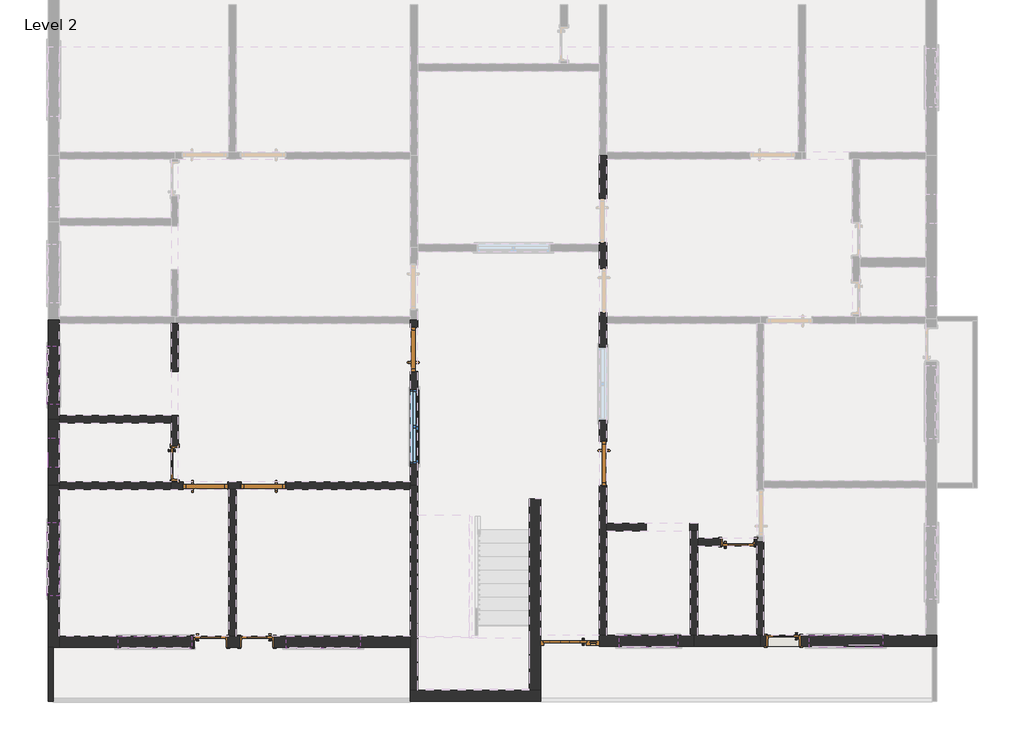
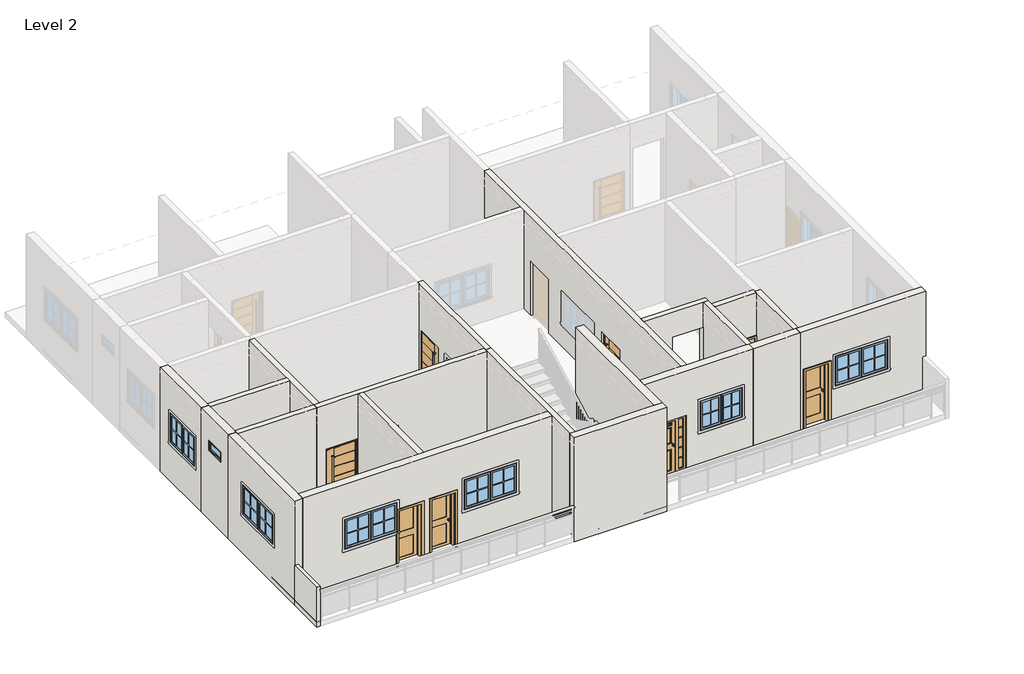
# One storey, part 1 of 5: 22 walls, 10 doors, 8 windows.
"""IFC4 building model written with IfcOpenShell, lengths in millimetres."""

from ifc_helpers import new_model, si_unit, frame, origin, place, context, project, spatial, polyline, outline, extrude, faceted_brep, transform, mapped, element, save
from components import door_3_ad1505b7, door_3_44036f4b, extsgl_w_side_panel_4_38b62cc9, door_c5a180fb, door_5f4ff63b, door_e2914254, fixed_2_d9cafb20, m_window_awning_double_horizontal_4_0c6a2509, m_window_awning_double_horizontal_5_7c720334, m_window_awning_double_horizontal_5_337400f2

model = new_model("IFC4")

# Units and contexts
model_context = context("Model", 3, world=origin())
ifc_project = project(units=[si_unit("LENGTHUNIT", "METRE", prefix="MILLI")], contexts=[model_context])

# Site, building, storey
site = spatial("IfcSite", under=ifc_project)
building = spatial("IfcBuilding", under=site)
storey = spatial("IfcBuildingStorey", under=building, Name="Level 2", Elevation=3200.4)

# Doors
placement = place(None, origin())
door_3_shape = door_3_ad1505b7(model_context)
element("IfcDoor", 1, ObjectType="3'", at=placement, inside=storey, context=model_context, shape_type="MappedRepresentation", body=[
    mapped(door_3_shape, transform((-17435.4847893, 15964.9922903, 3200.4), x_axis=(0.0, 1.0, 0.0), y_axis=(-1.0, 0.0, 0.0), z_axis=(0.0, 0.0, 1.0))),
])
element("IfcDoor", 2, ObjectType="3'", at=placement, inside=storey, context=model_context, shape_type="MappedRepresentation", body=[
    mapped(door_3_shape, transform((-20559.6847893, 13145.5922903, 3200.4), x_axis=(-1.0, 0.0, 0.0), y_axis=(0.0, -1.0, 0.0), z_axis=(0.0, 0.0, 1.0))),
])
element("IfcDoor", 3, ObjectType="3'", at=placement, inside=storey, context=model_context, shape_type="MappedRepresentation", body=[
    mapped(door_3_shape, transform((-13523.8847893, 13602.7922903, 3200.4), x_axis=(0.0, -1.0, 0.0), y_axis=(1.0, 0.0, 0.0), z_axis=(0.0, 0.0, 1.0))),
])
door_3_2_shape = door_3_44036f4b(model_context)
element("IfcDoor", 4, ObjectType="3'", at=placement, inside=storey, context=model_context, shape_type="MappedRepresentation", body=[
    mapped(door_3_2_shape, transform((-21753.4847893, 13145.5922903, 3200.4), x_axis=(1.0, 0.0, 0.0), y_axis=(0.0, 1.0, 0.0), z_axis=(0.0, 0.0, 1.0))),
])
extsgl_w_side_panel_4_shape = extsgl_w_side_panel_4_38b62cc9(model_context)
element("IfcDoor", 5, ObjectType="ExtSgl w Side Panel : 4'", at=placement, inside=storey, context=model_context, shape_type="MappedRepresentation", body=[
    mapped(extsgl_w_side_panel_4_shape, transform((-14429.0847893, 9932.4922903, 3200.4), x_axis=(-1.0, 0.0, 0.0), y_axis=(0.0, -1.0, 0.0), z_axis=(0.0, 0.0, 1.0))),
])
door_shape = door_c5a180fb(model_context)
element("IfcDoor", 6, ObjectType="M_Door-Interior-Single-2_Panel-Wood : 2'2\"", at=placement, inside=storey, context=model_context, shape_type="MappedRepresentation", body=[
    mapped(door_shape, transform((-22391.6597893, 13602.7922903, 3200.4), x_axis=(0.0, -1.0, 0.0), y_axis=(1.0, 0.0, 0.0), z_axis=(0.0, 0.0, 1.0))),
])
element("IfcDoor", 7, ObjectType="M_Door-Interior-Single-2_Panel-Wood : 2'2\"", at=placement, inside=storey, context=model_context, shape_type="MappedRepresentation", body=[
    mapped(door_shape, transform((-10729.8847893, 11974.0172903, 3200.4), x_axis=(1.0, 0.0, 0.0), y_axis=(0.0, 1.0, 0.0), z_axis=(0.0, 0.0, 1.0))),
])
door_2_shape = door_5f4ff63b(model_context)
element("IfcDoor", 8, ObjectType="M_Door-Interior-Single-2_Panel-Wood : 2'2\"", at=placement, inside=storey, context=model_context, shape_type="MappedRepresentation", body=[
    mapped(door_2_shape, transform((-21651.8847893, 9910.2672903, 3200.4), x_axis=(1.0, 0.0, 0.0), y_axis=(0.0, 1.0, 0.0), z_axis=(0.0, 0.0, 1.0))),
])
door_4_shape = door_e2914254(model_context)
element("IfcDoor", 9, ObjectType="M_Door-Interior-Single-2_Panel-Wood : 2'2\"", at=placement, inside=storey, context=model_context, shape_type="MappedRepresentation", body=[
    mapped(door_4_shape, transform((-20686.6847893, 9910.2672903, 3200.4), x_axis=(-1.0, 0.0, 0.0), y_axis=(0.0, -1.0, 0.0), z_axis=(0.0, 0.0, 1.0))),
])
element("IfcDoor", 10, ObjectType="M_Door-Interior-Single-2_Panel-Wood : 2'2\"", at=placement, inside=storey, context=model_context, shape_type="MappedRepresentation", body=[
    mapped(door_4_shape, transform((-9790.0847893, 9935.6672903, 3352.8), x_axis=(-1.0, 0.0, 0.0), y_axis=(0.0, -1.0, 0.0), z_axis=(0.0, 0.0, 1.0))),
])

# Walls
element("IfcWall", 11, ObjectType="Generic - 4\"", at=placement, inside=storey, context=model_context, shape_type="SweptSolid", body=[
    extrude(outline(polyline([(-25004.6847893, 8675.1922903), (-25004.6847893, 9792.7922903), (-24903.0847893, 9792.7922903), (-24903.0847893, 8675.1922903), (-25004.6847893, 8675.1922903)])), frame((0.0, 0.0, 3200.4), z_axis=(0.0, 0.0, 1.0), x_axis=(1.0, 0.0, 0.0)), (0.0, 0.0, 1.0), 1219.2),
])
element("IfcWall", 12, ObjectType="Generic - 6\"", at=placement, inside=storey, context=model_context, shape_type="Brep", body=[
    faceted_brep([(-24776.0847893, 13069.3922903, 3200.4), (-22477.3847893, 13069.3922903, 3200.4), (-22477.3847893, 13069.3922903, 6400.8), (-24776.0847893, 13069.3922903, 6400.8), (-24776.0847893, 13221.7922903, 3200.4), (-24776.0847893, 13221.7922903, 6400.8), (-22477.3847893, 13221.7922903, 6400.8), (-22477.3847893, 13221.7922903, 3200.4), (-24776.0847893, 13145.5922903, 3200.4), (-24776.0847893, 13145.5922903, 6400.8)], [[[0, 1, 2, 3]], [[4, 5, 6, 7]], [[1, 0, 8, 4, 7]], [[2, 1, 7, 6]], [[3, 2, 6, 5, 9]], [[0, 3, 9, 5, 4, 8]]]),
])
element("IfcWall", 13, ObjectType="Generic - 6\"", at=placement, inside=storey, context=model_context, shape_type="Brep", body=[
    faceted_brep([(-22464.6847893, 13221.7922903, 6400.8), (-22464.6847893, 14440.9922903, 6400.8), (-22464.6847893, 14593.3922903, 6400.8), (-22464.6847893, 16498.3922903, 6400.8), (-22464.6847893, 16498.3922903, 3200.4), (-22464.6847893, 15507.100075, 3200.4), (-22464.6847893, 15507.100075, 5638.8), (-22464.6847893, 14599.1617976, 5638.8), (-22464.6847893, 14599.1617976, 3200.4), (-22464.6847893, 14593.3922903, 3200.4), (-22464.6847893, 14440.9922903, 3200.4), (-22464.6847893, 13957.9922903, 3200.4), (-22464.6847893, 13957.9922903, 5054.2), (-22464.6847893, 13247.5922903, 5054.2), (-22464.6847893, 13247.5922903, 3200.4), (-22464.6847893, 13221.7922903, 3200.4), (-22312.2847893, 16498.3922903, 6400.8), (-22312.2847893, 13221.7922903, 6400.8), (-22312.2847893, 13221.7922903, 3200.4), (-22312.2847893, 13247.5922903, 3200.4), (-22312.2847893, 13247.5922903, 5054.2), (-22312.2847893, 13957.9922903, 5054.2), (-22312.2847893, 13957.9922903, 3200.4), (-22312.2847893, 14599.1617976, 3200.4), (-22312.2847893, 14599.1617976, 5638.8), (-22312.2847893, 15507.100075, 5638.8), (-22312.2847893, 15507.100075, 3200.4), (-22312.2847893, 16498.3922903, 3200.4), (-22388.4847893, 16498.3922903, 3200.4), (-22388.4847893, 16498.3922903, 6400.8)], [[[0, 1, 2, 3, 4, 5, 6, 7, 8, 9, 10, 11, 12, 13, 14, 15]], [[16, 17, 18, 19, 20, 21, 22, 23, 24, 25, 26, 27]], [[18, 15, 14, 19]], [[8, 23, 22, 11, 10, 9]], [[4, 28, 27, 26, 5]], [[3, 2, 1, 0, 17, 16, 29]], [[4, 3, 29, 16, 27, 28]], [[0, 15, 18, 17]], [[13, 20, 19, 14]], [[20, 13, 12, 21]], [[21, 12, 11, 22]], [[6, 25, 24, 7]], [[25, 6, 5, 26]], [[7, 24, 23, 8]]]),
])
element("IfcWall", 14, ObjectType="Generic - 6\"", at=placement, inside=storey, context=model_context, shape_type="Brep", body=[
    faceted_brep([(-24776.0847893, 14440.9922903, 3200.4), (-22464.6847893, 14440.9922903, 3200.4), (-22464.6847893, 14440.9922903, 6400.8), (-24776.0847893, 14440.9922903, 6400.8), (-24776.0847893, 14593.3922903, 3200.4), (-24776.0847893, 14593.3922903, 6400.8), (-22464.6847893, 14593.3922903, 6400.8), (-22464.6847893, 14593.3922903, 3200.4), (-24776.0847893, 14517.1922903, 3200.4), (-24776.0847893, 14517.1922903, 6400.8)], [[[0, 1, 2, 3]], [[4, 5, 6, 7]], [[1, 0, 8, 4, 7]], [[3, 2, 6, 5, 9]], [[0, 3, 9, 5, 4, 8]], [[2, 1, 7, 6]]]),
])
element("IfcWall", 15, ObjectType="Generic - 6\"", at=placement, inside=storey, context=model_context, shape_type="SweptSolid", body=[
    extrude(outline(polyline([(-21118.4847893, 13069.3922903), (-21118.4847893, 10021.3922903), (-21270.8847893, 10021.3922903), (-21270.8847893, 13069.3922903), (-21118.4847893, 13069.3922903)])), frame((0.0, 0.0, 3200.4), z_axis=(0.0, 0.0, 1.0), x_axis=(1.0, 0.0, 0.0)), (0.0, 0.0, 1.0), 3200.4),
])
element("IfcWall", 16, ObjectType="Generic - 6\"", at=placement, inside=storey, context=model_context, shape_type="Brep", body=[
    faceted_brep([(-11568.0847893, 12205.7922903, 3200.4), (-11568.0847893, 12205.7922903, 6400.8), (-11720.4847893, 12205.7922903, 6400.8), (-13447.6847893, 12205.7922903, 6400.8), (-13447.6847893, 12205.7922903, 3200.4), (-12628.6631671, 12205.7922903, 3200.4), (-12628.6631671, 12205.7922903, 5638.8), (-11726.8987952, 12205.7922903, 5638.8), (-11726.8987952, 12205.7922903, 3200.4), (-11720.4847893, 12205.7922903, 3200.4), (-11568.0847893, 12358.1922903, 6400.8), (-11568.0847893, 12358.1922903, 3200.4), (-11726.8987952, 12358.1922903, 3200.4), (-11726.8987952, 12358.1922903, 5638.8), (-12628.6631671, 12358.1922903, 5638.8), (-12628.6631671, 12358.1922903, 3200.4), (-13447.6847893, 12358.1922903, 3200.4), (-13447.6847893, 12358.1922903, 6400.8)], [[[0, 1, 2, 3, 4, 5, 6, 7, 8, 9]], [[10, 11, 12, 13, 14, 15, 16, 17]], [[4, 16, 15, 5]], [[11, 0, 9, 8, 12]], [[3, 2, 1, 10, 17]], [[4, 3, 17, 16]], [[1, 0, 11, 10]], [[6, 14, 13, 7]], [[14, 6, 5, 15]], [[7, 13, 12, 8]]]),
])
element("IfcWall", 17, ObjectType="Generic - 6\"", at=placement, inside=storey, context=model_context, shape_type="Brep", body=[
    faceted_brep([(-11720.4847893, 12205.7922903, 3200.4), (-11720.4847893, 10046.7922903, 3200.4), (-11720.4847893, 10046.7922903, 6400.8), (-11720.4847893, 12205.7922903, 6400.8), (-11568.0847893, 12205.7922903, 3200.4), (-11568.0847893, 12205.7922903, 6400.8), (-11568.0847893, 12053.3922903, 6400.8), (-11568.0847893, 11900.9922903, 6400.8), (-11568.0847893, 10046.7922903, 6400.8), (-11568.0847893, 10046.7922903, 3200.4), (-11568.0847893, 11900.9922903, 3200.4), (-11568.0847893, 12053.3922903, 3200.4), (-11644.2847893, 10046.7922903, 3200.4), (-11644.2847893, 10046.7922903, 6400.8)], [[[0, 1, 2, 3]], [[4, 5, 6, 7, 8, 9, 10, 11]], [[1, 0, 4, 11, 10, 9, 12]], [[3, 2, 13, 8, 7, 6, 5]], [[0, 3, 5, 4]], [[2, 1, 12, 9, 8, 13]]]),
])
element("IfcWall", 18, ObjectType="Generic - 6\"", at=placement, inside=storey, context=model_context, shape_type="Brep", body=[
    faceted_brep([(-10348.8847893, 11900.9922903, 6400.8), (-11568.0847893, 11900.9922903, 6400.8), (-11568.0847893, 11900.9922903, 3200.4), (-11085.0847893, 11900.9922903, 3200.4), (-11085.0847893, 11900.9922903, 5054.2), (-10374.6847893, 11900.9922903, 5054.2), (-10374.6847893, 11900.9922903, 3200.4), (-10348.8847893, 11900.9922903, 3200.4), (-11568.0847893, 12053.3922903, 6400.8), (-10348.8847893, 12053.3922903, 6400.8), (-10348.8847893, 12053.3922903, 3200.4), (-10374.6847893, 12053.3922903, 3200.4), (-10374.6847893, 12053.3922903, 5054.2), (-11085.0847893, 12053.3922903, 5054.2), (-11085.0847893, 12053.3922903, 3200.4), (-11568.0847893, 12053.3922903, 3200.4), (-10348.8847893, 11977.1922903, 3200.4), (-10348.8847893, 11977.1922903, 6400.8)], [[[0, 1, 2, 3, 4, 5, 6, 7]], [[8, 9, 10, 11, 12, 13, 14, 15]], [[2, 15, 14, 3]], [[10, 16, 7, 6, 11]], [[1, 0, 17, 9, 8]], [[2, 1, 8, 15]], [[5, 12, 11, 6]], [[12, 5, 4, 13]], [[13, 4, 3, 14]], [[0, 7, 16, 10, 9, 17]]]),
])
element("IfcWall", 19, ObjectType="Generic - 6\"", at=placement, inside=storey, context=model_context, shape_type="Brep", body=[
    faceted_brep([(-13600.0847893, 10046.7922903, 6400.8), (-13600.0847893, 17996.9922903, 6400.8), (-13600.0847893, 18149.3922903, 6400.8), (-13600.0847893, 19978.1922903, 6400.8), (-13600.0847893, 19978.1922903, 3200.4), (-13600.0847893, 19089.1922903, 3200.4), (-13600.0847893, 19089.1922903, 5029.2), (-13600.0847893, 18174.7922903, 5029.2), (-13600.0847893, 18174.7922903, 3200.4), (-13600.0847893, 18149.3922903, 3200.4), (-13600.0847893, 17996.9922903, 3200.4), (-13600.0847893, 17641.3922903, 3200.4), (-13600.0847893, 17641.3922903, 5029.2), (-13600.0847893, 16726.9922903, 5029.2), (-13600.0847893, 16726.9922903, 3200.4), (-13600.0847893, 14059.9922903, 3200.4), (-13600.0847893, 14059.9922903, 5029.2), (-13600.0847893, 13145.5922903, 5029.2), (-13600.0847893, 13145.5922903, 3200.4), (-13600.0847893, 10046.7922903, 3200.4), (-13600.0847893, 10046.7922903, 5029.2), (-13600.0847893, 16015.7922903, 5014.8), (-13600.0847893, 14491.7922903, 5014.8), (-13600.0847893, 14491.7922903, 4100.4), (-13600.0847893, 16015.7922903, 4100.4), (-13447.6847893, 19978.1922903, 6400.8), (-13447.6847893, 19901.9922903, 6400.8), (-13447.6847893, 16650.7922903, 6400.8), (-13447.6847893, 16498.3922903, 6400.8), (-13447.6847893, 12358.1922903, 6400.8), (-13447.6847893, 12205.7922903, 6400.8), (-13447.6847893, 10046.7922903, 6400.8), (-13447.6847893, 10046.7922903, 3200.4), (-13447.6847893, 12205.7922903, 3200.4), (-13447.6847893, 12358.1922903, 3200.4), (-13447.6847893, 13145.5922903, 3200.4), (-13447.6847893, 13145.5922903, 5029.2), (-13447.6847893, 14059.9922903, 5029.2), (-13447.6847893, 14059.9922903, 3200.4), (-13447.6847893, 16498.3922903, 3200.4), (-13447.6847893, 16650.7922903, 3200.4), (-13447.6847893, 16726.9922903, 3200.4), (-13447.6847893, 16726.9922903, 5029.2), (-13447.6847893, 17641.3922903, 5029.2), (-13447.6847893, 17641.3922903, 3200.4), (-13447.6847893, 18174.7922903, 3200.4), (-13447.6847893, 18174.7922903, 5029.2), (-13447.6847893, 19089.1922903, 5029.2), (-13447.6847893, 19089.1922903, 3200.4), (-13447.6847893, 19901.9922903, 3200.4), (-13447.6847893, 19978.1922903, 3200.4), (-13447.6847893, 16015.7922903, 5014.8), (-13447.6847893, 16015.7922903, 4100.4), (-13447.6847893, 14491.7922903, 4100.4), (-13447.6847893, 14491.7922903, 5014.8), (-13544.6847893, 13145.5922903, 3200.4), (-13544.6847893, 13130.5922903, 3200.4), (-13467.6847893, 13130.5922903, 3200.4), (-13467.6847893, 13145.5922903, 3200.4), (-13544.6847893, 14059.9922903, 3200.4), (-13544.6847893, 16726.9922903, 3200.4), (-13544.6847893, 16711.9922903, 3200.4), (-13467.6847893, 16711.9922903, 3200.4), (-13467.6847893, 16726.9922903, 3200.4), (-13467.6847893, 14059.9922903, 3200.4), (-13467.6847893, 14074.9922903, 3200.4), (-13544.6847893, 14074.9922903, 3200.4), (-13544.6847893, 17641.3922903, 3200.4), (-13580.0847893, 18174.7922903, 3200.4), (-13580.0847893, 18159.7922903, 3200.4), (-13503.0847893, 18159.7922903, 3200.4), (-13503.0847893, 18174.7922903, 3200.4), (-13467.6847893, 17641.3922903, 3200.4), (-13467.6847893, 17656.3922903, 3200.4), (-13544.6847893, 17656.3922903, 3200.4), (-13503.0847893, 19089.1922903, 3200.4), (-13503.0847893, 19104.1922903, 3200.4), (-13580.0847893, 19104.1922903, 3200.4), (-13580.0847893, 19089.1922903, 3200.4), (-13544.6847893, 14059.9922903, 5029.2), (-13544.6847893, 13145.5922903, 5029.2), (-13467.6847893, 14059.9922903, 5029.2), (-13467.6847893, 13145.5922903, 5029.2), (-13467.6847893, 14074.9922903, 5044.2), (-13467.6847893, 13130.5922903, 5044.2), (-13544.6847893, 13130.5922903, 5044.2), (-13544.6847893, 14074.9922903, 5044.2), (-13544.6847893, 17641.3922903, 5029.2), (-13544.6847893, 16726.9922903, 5029.2), (-13467.6847893, 17641.3922903, 5029.2), (-13467.6847893, 16726.9922903, 5029.2), (-13467.6847893, 17656.3922903, 5044.2), (-13467.6847893, 16711.9922903, 5044.2), (-13544.6847893, 16711.9922903, 5044.2), (-13544.6847893, 17656.3922903, 5044.2), (-13580.0847893, 19089.1922903, 5029.2), (-13580.0847893, 18174.7922903, 5029.2), (-13503.0847893, 18174.7922903, 5029.2), (-13503.0847893, 19089.1922903, 5029.2), (-13580.0847893, 19104.1922903, 5044.2), (-13503.0847893, 19104.1922903, 5044.2), (-13503.0847893, 18159.7922903, 5044.2), (-13580.0847893, 18159.7922903, 5044.2)], [[[0, 1, 2, 3, 4, 5, 6, 7, 8, 9, 10, 11, 12, 13, 14, 15, 16, 17, 18, 19, 20], [21, 22, 23, 24]], [[25, 26, 27, 28, 29, 30, 31, 32, 33, 34, 35, 36, 37, 38, 39, 40, 41, 42, 43, 44, 45, 46, 47, 48, 49, 50], [51, 52, 53, 54]], [[32, 19, 18, 55, 56, 57, 58, 35, 34, 33]], [[59, 15, 14, 60, 61, 62, 63, 41, 40, 39, 38, 64, 65, 66]], [[67, 11, 10, 9, 8, 68, 69, 70, 71, 45, 44, 72, 73, 74]], [[4, 50, 49, 48, 75, 76, 77, 78, 5]], [[3, 2, 1, 0, 31, 30, 29, 28, 27, 26, 25]], [[4, 3, 25, 50]], [[0, 20, 19, 32, 31]], [[16, 79, 80, 17]], [[81, 37, 36, 82]], [[17, 80, 55, 18]], [[82, 36, 35, 58]], [[79, 16, 15, 59]], [[37, 81, 64, 38]], [[83, 84, 85, 86]], [[85, 84, 57, 56]], [[86, 85, 56, 55, 80, 79, 59, 66]], [[83, 86, 66, 65]], [[84, 83, 65, 64, 81, 82, 58, 57]], [[12, 87, 88, 13]], [[89, 43, 42, 90]], [[13, 88, 60, 14]], [[90, 42, 41, 63]], [[87, 12, 11, 67]], [[43, 89, 72, 44]], [[91, 92, 93, 94]], [[93, 92, 62, 61]], [[94, 93, 61, 60, 88, 87, 67, 74]], [[91, 94, 74, 73]], [[92, 91, 73, 72, 89, 90, 63, 62]], [[6, 95, 96, 7]], [[46, 97, 98, 47]], [[97, 46, 45, 71]], [[7, 96, 68, 8]], [[47, 98, 75, 48]], [[95, 6, 5, 78]], [[99, 100, 101, 102]], [[102, 101, 70, 69]], [[98, 97, 71, 70, 101, 100, 76, 75]], [[100, 99, 77, 76]], [[96, 95, 78, 77, 99, 102, 69, 68]], [[51, 54, 22, 21]], [[54, 53, 23, 22]], [[53, 52, 24, 23]], [[52, 51, 21, 24]]]),
])
element("IfcWall", 20, ObjectType="Generic - 6\"", at=placement, inside=storey, context=model_context, shape_type="Brep", body=[
    faceted_brep([(-17511.6847893, 13145.5922903, 3200.4), (-17511.6847893, 13145.5922903, 6400.8), (-17511.6847893, 13221.7922903, 6400.8), (-17511.6847893, 16498.3922903, 6400.8), (-17511.6847893, 16574.5922903, 6400.8), (-17511.6847893, 16574.5922903, 3200.4), (-17511.6847893, 16498.3922903, 3200.4), (-17511.6847893, 16422.1922903, 3200.4), (-17511.6847893, 16422.1922903, 5029.2), (-17511.6847893, 15507.7922903, 5029.2), (-17511.6847893, 15507.7922903, 3200.4), (-17511.6847893, 13221.7922903, 3200.4), (-17511.6847893, 13602.7922903, 5014.8), (-17511.6847893, 13602.7922903, 4100.4), (-17511.6847893, 15126.7922903, 4100.4), (-17511.6847893, 15126.7922903, 5014.8), (-17359.2847893, 13145.5922903, 6400.8), (-17359.2847893, 13145.5922903, 3200.4), (-17359.2847893, 15507.7922903, 3200.4), (-17359.2847893, 15507.7922903, 5029.2), (-17359.2847893, 16422.1922903, 5029.2), (-17359.2847893, 16422.1922903, 3200.4), (-17359.2847893, 16574.5922903, 3200.4), (-17359.2847893, 16574.5922903, 6400.8), (-17359.2847893, 13602.7922903, 5014.8), (-17359.2847893, 15126.7922903, 5014.8), (-17359.2847893, 15126.7922903, 4100.4), (-17359.2847893, 13602.7922903, 4100.4), (-17414.6847893, 16422.1922903, 3200.4), (-17414.6847893, 16437.1922903, 3200.4), (-17491.6847893, 16437.1922903, 3200.4), (-17491.6847893, 16422.1922903, 3200.4), (-17491.6847893, 15507.7922903, 3200.4), (-17491.6847893, 15492.7922903, 3200.4), (-17414.6847893, 15492.7922903, 3200.4), (-17414.6847893, 15507.7922903, 3200.4), (-17414.6847893, 15507.7922903, 5029.2), (-17414.6847893, 16422.1922903, 5029.2), (-17491.6847893, 16422.1922903, 5029.2), (-17491.6847893, 15507.7922903, 5029.2), (-17491.6847893, 15492.7922903, 5044.2), (-17491.6847893, 16437.1922903, 5044.2), (-17414.6847893, 16437.1922903, 5044.2), (-17414.6847893, 15492.7922903, 5044.2)], [[[0, 1, 2, 3, 4, 5, 6, 7, 8, 9, 10, 11], [12, 13, 14, 15]], [[16, 17, 18, 19, 20, 21, 22, 23], [24, 25, 26, 27]], [[5, 22, 21, 28, 29, 30, 31, 7, 6]], [[17, 0, 11, 10, 32, 33, 34, 35, 18]], [[1, 0, 17, 16]], [[4, 3, 2, 1, 16, 23]], [[5, 4, 23, 22]], [[19, 36, 37, 20]], [[8, 38, 39, 9]], [[20, 37, 28, 21]], [[38, 8, 7, 31]], [[36, 19, 18, 35]], [[9, 39, 32, 10]], [[40, 41, 42, 43]], [[42, 41, 30, 29]], [[37, 36, 35, 34, 43, 42, 29, 28]], [[40, 43, 34, 33]], [[39, 38, 31, 30, 41, 40, 33, 32]], [[12, 15, 25, 24]], [[15, 14, 26, 25]], [[14, 13, 27, 26]], [[13, 12, 24, 27]]]),
])
element("IfcWall", 21, ObjectType="Generic - 6\"", at=placement, inside=storey, context=model_context, shape_type="Brep", body=[
    faceted_brep([(-17511.6847893, 13145.5922903, 3200.4), (-17511.6847893, 13069.3922903, 3200.4), (-17511.6847893, 10021.3922903, 3200.4), (-17511.6847893, 9792.7922903, 3200.4), (-17511.6847893, 8903.7922903, 3200.4), (-17511.6847893, 8903.7922903, 6400.8), (-17511.6847893, 9792.7922903, 6400.8), (-17511.6847893, 10021.3922903, 6400.8), (-17511.6847893, 13069.3922903, 6400.8), (-17511.6847893, 13145.5922903, 6400.8), (-17359.2847893, 13145.5922903, 3200.4), (-17359.2847893, 13145.5922903, 6400.8), (-17359.2847893, 8903.7922903, 6400.8), (-17359.2847893, 8903.7922903, 3200.4)], [[[0, 1, 2, 3, 4, 5, 6, 7, 8, 9]], [[10, 11, 12, 13]], [[4, 3, 2, 1, 0, 10, 13]], [[9, 8, 7, 6, 5, 12, 11]], [[0, 9, 11, 10]], [[5, 4, 13, 12]]]),
])
element("IfcWall", 22, ObjectType="Generic - 6\"", at=placement, inside=storey, context=model_context, shape_type="Brep", body=[
    faceted_brep([(-17511.6847893, 13069.3922903, 6400.8), (-21118.4847893, 13069.3922903, 6400.8), (-21270.8847893, 13069.3922903, 6400.8), (-22477.3847893, 13069.3922903, 6400.8), (-22477.3847893, 13069.3922903, 3200.4), (-22210.6847893, 13069.3922903, 3200.4), (-22210.6847893, 13069.3922903, 5029.2), (-21296.2847893, 13069.3922903, 5029.2), (-21296.2847893, 13069.3922903, 3200.4), (-21270.8847893, 13069.3922903, 3200.4), (-21118.4847893, 13069.3922903, 3200.4), (-21016.8847893, 13069.3922903, 3200.4), (-21016.8847893, 13069.3922903, 5029.2), (-20102.4847893, 13069.3922903, 5029.2), (-20102.4847893, 13069.3922903, 3200.4), (-17511.6847893, 13069.3922903, 3200.4), (-22477.3847893, 13221.7922903, 6400.8), (-22464.6847893, 13221.7922903, 6400.8), (-22312.2847893, 13221.7922903, 6400.8), (-17511.6847893, 13221.7922903, 6400.8), (-17511.6847893, 13221.7922903, 3200.4), (-20102.4847893, 13221.7922903, 3200.4), (-20102.4847893, 13221.7922903, 5029.2), (-21016.8847893, 13221.7922903, 5029.2), (-21016.8847893, 13221.7922903, 3200.4), (-21296.2847893, 13221.7922903, 3200.4), (-21296.2847893, 13221.7922903, 5029.2), (-22210.6847893, 13221.7922903, 5029.2), (-22210.6847893, 13221.7922903, 3200.4), (-22312.2847893, 13221.7922903, 3200.4), (-22464.6847893, 13221.7922903, 3200.4), (-22477.3847893, 13221.7922903, 3200.4), (-17511.6847893, 13145.5922903, 3200.4), (-20102.4847893, 13089.3922903, 3200.4), (-20087.4847893, 13089.3922903, 3200.4), (-20087.4847893, 13166.3922903, 3200.4), (-20102.4847893, 13166.3922903, 3200.4), (-21296.2847893, 13089.3922903, 3200.4), (-21281.2847893, 13089.3922903, 3200.4), (-21281.2847893, 13166.3922903, 3200.4), (-21296.2847893, 13166.3922903, 3200.4), (-21016.8847893, 13166.3922903, 3200.4), (-21031.8847893, 13166.3922903, 3200.4), (-21031.8847893, 13089.3922903, 3200.4), (-21016.8847893, 13089.3922903, 3200.4), (-22210.6847893, 13166.3922903, 3200.4), (-22225.6847893, 13166.3922903, 3200.4), (-22225.6847893, 13089.3922903, 3200.4), (-22210.6847893, 13089.3922903, 3200.4), (-17511.6847893, 13145.5922903, 6400.8), (-22210.6847893, 13166.3922903, 5029.2), (-21296.2847893, 13166.3922903, 5029.2), (-22210.6847893, 13089.3922903, 5029.2), (-21296.2847893, 13089.3922903, 5029.2), (-21281.2847893, 13089.3922903, 5044.2), (-22225.6847893, 13089.3922903, 5044.2), (-22225.6847893, 13166.3922903, 5044.2), (-21281.2847893, 13166.3922903, 5044.2), (-20102.4847893, 13166.3922903, 5029.2), (-21016.8847893, 13166.3922903, 5029.2), (-21016.8847893, 13089.3922903, 5029.2), (-20102.4847893, 13089.3922903, 5029.2), (-20087.4847893, 13089.3922903, 5044.2), (-21031.8847893, 13089.3922903, 5044.2), (-21031.8847893, 13166.3922903, 5044.2), (-20087.4847893, 13166.3922903, 5044.2)], [[[0, 1, 2, 3, 4, 5, 6, 7, 8, 9, 10, 11, 12, 13, 14, 15]], [[16, 17, 18, 19, 20, 21, 22, 23, 24, 25, 26, 27, 28, 29, 30, 31]], [[20, 32, 15, 14, 33, 34, 35, 36, 21]], [[8, 37, 38, 39, 40, 25, 24, 41, 42, 43, 44, 11, 10, 9]], [[4, 31, 30, 29, 28, 45, 46, 47, 48, 5]], [[3, 2, 1, 0, 49, 19, 18, 17, 16]], [[4, 3, 16, 31]], [[0, 15, 32, 20, 19, 49]], [[50, 27, 26, 51]], [[6, 52, 53, 7]], [[51, 26, 25, 40]], [[7, 53, 37, 8]], [[27, 50, 45, 28]], [[52, 6, 5, 48]], [[54, 55, 56, 57]], [[54, 57, 39, 38]], [[57, 56, 46, 45, 50, 51, 40, 39]], [[56, 55, 47, 46]], [[55, 54, 38, 37, 53, 52, 48, 47]], [[22, 58, 59, 23]], [[12, 60, 61, 13]], [[23, 59, 41, 24]], [[60, 12, 11, 44]], [[58, 22, 21, 36]], [[13, 61, 33, 14]], [[62, 63, 64, 65]], [[64, 63, 43, 42]], [[59, 58, 36, 35, 65, 64, 42, 41]], [[62, 65, 35, 34]], [[61, 60, 44, 43, 63, 62, 34, 33]]]),
])
element("IfcWall", 23, ObjectType="Generic - 6\"", at=placement, inside=storey, context=model_context, shape_type="Brep", body=[
    faceted_brep([(-10348.8847893, 11977.1922903, 3200.4), (-10348.8847893, 11900.9922903, 3200.4), (-10348.8847893, 10046.7922903, 3200.4), (-10348.8847893, 10046.7922903, 6400.8), (-10348.8847893, 11900.9922903, 6400.8), (-10348.8847893, 11977.1922903, 6400.8), (-10196.4847893, 11977.1922903, 3200.4), (-10196.4847893, 11977.1922903, 6400.8), (-10196.4847893, 10046.7922903, 6400.8), (-10196.4847893, 10046.7922903, 3200.4), (-10272.6847893, 10046.7922903, 3200.4), (-10272.6847893, 10046.7922903, 6400.8)], [[[0, 1, 2, 3, 4, 5]], [[6, 7, 8, 9]], [[2, 1, 0, 6, 9, 10]], [[5, 4, 3, 11, 8, 7]], [[0, 5, 7, 6]], [[3, 2, 10, 9, 8, 11]]]),
])
element("IfcWall", 24, ObjectType="Generic - 9\"", at=placement, inside=storey, context=model_context, shape_type="Brep", body=[
    faceted_brep([(-17511.6847893, 9792.7922903, 6400.8), (-24776.0847893, 9792.7922903, 6400.8), (-24776.0847893, 9792.7922903, 3200.4), (-22007.0847893, 9792.7922903, 3200.4), (-22007.0847893, 9792.7922903, 5054.2), (-21296.6847893, 9792.7922903, 5054.2), (-21296.6847893, 9792.7922903, 3200.4), (-21041.8847893, 9792.7922903, 3200.4), (-21041.8847893, 9792.7922903, 5054.2), (-20331.4847893, 9792.7922903, 5054.2), (-20331.4847893, 9792.7922903, 3200.4), (-17511.6847893, 9792.7922903, 3200.4), (-23556.8847893, 9792.7922903, 5333.9570313), (-22032.8847893, 9792.7922903, 5333.9570313), (-22032.8847893, 9792.7922903, 4419.5570313), (-23556.8847893, 9792.7922903, 4419.5570313), (-20077.0847893, 9792.7922903, 5333.9570313), (-18553.0847893, 9792.7922903, 5333.9570313), (-18553.0847893, 9792.7922903, 4419.5570313), (-20077.0847893, 9792.7922903, 4419.5570313), (-24776.0847893, 10021.3922903, 6400.8), (-21270.8847893, 10021.3922903, 6400.8), (-21118.4847893, 10021.3922903, 6400.8), (-17511.6847893, 10021.3922903, 6400.8), (-17511.6847893, 10021.3922903, 3200.4), (-20331.4847893, 10021.3922903, 3200.4), (-20331.4847893, 10021.3922903, 5054.2), (-21041.8847893, 10021.3922903, 5054.2), (-21041.8847893, 10021.3922903, 3200.4), (-21118.4847893, 10021.3922903, 3200.4), (-21270.8847893, 10021.3922903, 3200.4), (-21296.6847893, 10021.3922903, 3200.4), (-21296.6847893, 10021.3922903, 5054.2), (-22007.0847893, 10021.3922903, 5054.2), (-22007.0847893, 10021.3922903, 3200.4), (-24776.0847893, 10021.3922903, 3200.4), (-23556.8847893, 10021.3922903, 5333.9570313), (-23556.8847893, 10021.3922903, 4419.5570313), (-22032.8847893, 10021.3922903, 4419.5570313), (-22032.8847893, 10021.3922903, 5333.9570313), (-20077.0847893, 10021.3922903, 5333.9570313), (-20077.0847893, 10021.3922903, 4419.5570313), (-18553.0847893, 10021.3922903, 4419.5570313), (-18553.0847893, 10021.3922903, 5333.9570313)], [[[0, 1, 2, 3, 4, 5, 6, 7, 8, 9, 10, 11], [12, 13, 14, 15], [16, 17, 18, 19]], [[20, 21, 22, 23, 24, 25, 26, 27, 28, 29, 30, 31, 32, 33, 34, 35], [36, 37, 38, 39], [40, 41, 42, 43]], [[2, 35, 34, 3]], [[24, 11, 10, 25]], [[6, 31, 30, 29, 28, 7]], [[1, 0, 23, 22, 21, 20]], [[0, 11, 24, 23]], [[37, 36, 12, 15]], [[38, 37, 15, 14]], [[39, 38, 14, 13]], [[36, 39, 13, 12]], [[41, 40, 16, 19]], [[42, 41, 19, 18]], [[43, 42, 18, 17]], [[40, 43, 17, 16]], [[6, 5, 32, 31]], [[5, 4, 33, 32]], [[4, 3, 34, 33]], [[27, 8, 7, 28]], [[8, 27, 26, 9]], [[9, 26, 25, 10]], [[1, 20, 35, 2]]]),
])
element("IfcWall", 25, ObjectType="Generic - 9\"", at=placement, inside=storey, context=model_context, shape_type="Brep", body=[
    faceted_brep([(-17511.6847893, 8675.1922903, 3200.4), (-14819.2847893, 8675.1922903, 3200.4), (-14819.2847893, 8675.1922903, 6400.8), (-17511.6847893, 8675.1922903, 6400.8), (-17511.6847893, 8903.7922903, 3200.4), (-17511.6847893, 8903.7922903, 6400.8), (-17359.2847893, 8903.7922903, 6400.8), (-15047.8847893, 8903.7922903, 6400.8), (-14819.2847893, 8903.7922903, 6400.8), (-14819.2847893, 8903.7922903, 3200.4), (-15047.8847893, 8903.7922903, 3200.4), (-17359.2847893, 8903.7922903, 3200.4)], [[[0, 1, 2, 3]], [[4, 5, 6, 7, 8, 9, 10, 11]], [[1, 0, 4, 11, 10, 9]], [[3, 2, 8, 7, 6, 5]], [[2, 1, 9, 8]], [[0, 3, 5, 4]]]),
])
element("IfcWall", 26, ObjectType="Generic - 9\"", at=placement, inside=storey, context=model_context, shape_type="Brep", body=[
    faceted_brep([(-14819.2847893, 8903.7922903, 3200.4), (-14819.2847893, 12866.1922903, 3200.4), (-14819.2847893, 12866.1922903, 6400.8), (-14819.2847893, 10046.7922903, 6400.8), (-14819.2847893, 9818.1922903, 6400.8), (-14819.2847893, 8903.7922903, 6400.8), (-15047.8847893, 8903.7922903, 3200.4), (-15047.8847893, 8903.7922903, 6400.8), (-15047.8847893, 12866.1922903, 6400.8), (-15047.8847893, 12866.1922903, 3200.4)], [[[0, 1, 2, 3, 4, 5]], [[6, 7, 8, 9]], [[1, 0, 6, 9]], [[2, 1, 9, 8]], [[5, 4, 3, 2, 8, 7]], [[0, 5, 7, 6]]]),
])
element("IfcWall", 27, ObjectType="Generic - 9\"", at=placement, inside=storey, context=model_context, shape_type="Brep", body=[
    faceted_brep([(-6615.0847893, 10046.7922903, 3200.4), (-6843.6847893, 10046.7922903, 3200.4), (-10196.4847893, 10046.7922903, 3200.4), (-10272.6847893, 10046.7922903, 3200.4), (-10272.6847893, 10046.7922903, 6400.8), (-10196.4847893, 10046.7922903, 6400.8), (-6843.6847893, 10046.7922903, 6400.8), (-6615.0847893, 10046.7922903, 6400.8), (-9263.0347893, 10046.7922903, 5333.9570313), (-9263.0347893, 10046.7922903, 4419.5570313), (-7739.0347893, 10046.7922903, 4419.5570313), (-7739.0347893, 10046.7922903, 5333.9570313), (-10145.2847893, 10046.7922903, 5206.6), (-10145.2847893, 10046.7922903, 3352.8), (-9434.8847893, 10046.7922903, 3352.8), (-9434.8847893, 10046.7922903, 5206.6), (-10272.6847893, 9818.1922903, 3200.4), (-6716.6847893, 9818.1922903, 3200.4), (-6615.0847893, 9818.1922903, 3200.4), (-6615.0847893, 9818.1922903, 4419.6), (-6615.0847893, 9818.1922903, 6400.8), (-10272.6847893, 9818.1922903, 6400.8), (-9263.0347893, 9818.1922903, 5333.9570313), (-7739.0347893, 9818.1922903, 5333.9570313), (-7739.0347893, 9818.1922903, 4419.5570313), (-9263.0347893, 9818.1922903, 4419.5570313), (-10145.2847893, 9818.1922903, 3352.8), (-10145.2847893, 9818.1922903, 5206.6), (-9434.8847893, 9818.1922903, 5206.6), (-9434.8847893, 9818.1922903, 3352.8)], [[[0, 1, 2, 3, 4, 5, 6, 7], [8, 9, 10, 11], [12, 13, 14, 15]], [[16, 17, 18, 19, 20, 21], [22, 23, 24, 25], [26, 27, 28, 29]], [[3, 2, 1, 0, 18, 17, 16]], [[4, 3, 16, 21]], [[7, 6, 5, 4, 21, 20]], [[9, 8, 22, 25]], [[10, 9, 25, 24]], [[11, 10, 24, 23]], [[8, 11, 23, 22]], [[26, 13, 12, 27]], [[27, 12, 15, 28]], [[28, 15, 14, 29]], [[13, 26, 29, 14]], [[7, 20, 19, 18, 0]]]),
])
element("IfcWall", 28, ObjectType="Generic - 9\"", at=placement, inside=storey, context=model_context, shape_type="Brep", body=[
    faceted_brep([(-10272.6847893, 10046.7922903, 3200.4), (-10348.8847893, 10046.7922903, 3200.4), (-11568.0847893, 10046.7922903, 3200.4), (-11644.2847893, 10046.7922903, 3200.4), (-11644.2847893, 10046.7922903, 6400.8), (-11568.0847893, 10046.7922903, 6400.8), (-10348.8847893, 10046.7922903, 6400.8), (-10272.6847893, 10046.7922903, 6400.8), (-10272.6847893, 9818.1922903, 3200.4), (-10272.6847893, 9818.1922903, 6400.8), (-11644.2847893, 9818.1922903, 6400.8), (-11644.2847893, 9818.1922903, 3200.4)], [[[0, 1, 2, 3, 4, 5, 6, 7]], [[8, 9, 10, 11]], [[3, 2, 1, 0, 8, 11]], [[4, 3, 11, 10]], [[7, 6, 5, 4, 10, 9]], [[0, 7, 9, 8]]]),
])
element("IfcWall", 29, ObjectType="Generic - 9\"", at=placement, inside=storey, context=model_context, shape_type="Brep", body=[
    faceted_brep([(-14819.2847893, 10046.7922903, 6400.8), (-13600.0847893, 10046.7922903, 6400.8), (-13447.6847893, 10046.7922903, 6400.8), (-11720.4847893, 10046.7922903, 6400.8), (-11644.2847893, 10046.7922903, 6400.8), (-11644.2847893, 10046.7922903, 3200.4), (-11720.4847893, 10046.7922903, 3200.4), (-13447.6847893, 10046.7922903, 3200.4), (-13600.0847893, 10046.7922903, 3200.4), (-13600.0847893, 10046.7922903, 5029.2), (-14819.2847893, 10046.7922903, 5029.2), (-13193.6847893, 10046.7922903, 5334.0), (-13193.6847893, 10046.7922903, 4419.6), (-11974.4847893, 10046.7922903, 4419.6), (-11974.4847893, 10046.7922903, 5334.0), (-11644.2847893, 9818.1922903, 6400.8), (-14819.2847893, 9818.1922903, 6400.8), (-14819.2847893, 9818.1922903, 5029.2), (-13600.0847893, 9818.1922903, 5029.2), (-13600.0847893, 9818.1922903, 3200.4), (-11644.2847893, 9818.1922903, 3200.4), (-13193.6847893, 9818.1922903, 5334.0), (-11974.4847893, 9818.1922903, 5334.0), (-11974.4847893, 9818.1922903, 4419.6), (-13193.6847893, 9818.1922903, 4419.6)], [[[0, 1, 2, 3, 4, 5, 6, 7, 8, 9, 10], [11, 12, 13, 14]], [[15, 16, 17, 18, 19, 20], [21, 22, 23, 24]], [[5, 20, 19, 8, 7, 6]], [[4, 3, 2, 1, 0, 16, 15]], [[5, 4, 15, 20]], [[16, 0, 10, 17]], [[11, 14, 22, 21]], [[14, 13, 23, 22]], [[13, 12, 24, 23]], [[12, 11, 21, 24]], [[18, 9, 8, 19]], [[9, 18, 17, 10]]]),
])
element("IfcWall", 30, ObjectType="Generic - 9\"", at=placement, inside=storey, context=model_context, shape_type="Brep", body=[
    faceted_brep([(-25004.6847893, 16574.5922903, 3200.4), (-25004.6847893, 14517.1922903, 3200.4), (-25004.6847893, 14517.1922903, 6400.8), (-25004.6847893, 16574.5922903, 6400.8), (-25004.6847893, 16041.1922903, 5334.0), (-25004.6847893, 14821.9922903, 5334.0), (-25004.6847893, 14821.9922903, 4419.6), (-25004.6847893, 16041.1922903, 4419.6), (-24776.0847893, 16574.5922903, 3200.4), (-24776.0847893, 16574.5922903, 6400.8), (-24776.0847893, 16498.3922903, 6400.8), (-24776.0847893, 14593.3922903, 6400.8), (-24776.0847893, 14517.1922903, 6400.8), (-24776.0847893, 14517.1922903, 3200.4), (-24776.0847893, 14593.3922903, 3200.4), (-24776.0847893, 16498.3922903, 3200.4), (-24776.0847893, 16041.1922903, 5334.0), (-24776.0847893, 16041.1922903, 4419.6), (-24776.0847893, 14821.9922903, 4419.6), (-24776.0847893, 14821.9922903, 5334.0)], [[[0, 1, 2, 3], [4, 5, 6, 7]], [[8, 9, 10, 11, 12, 13, 14, 15], [16, 17, 18, 19]], [[1, 0, 8, 15, 14, 13]], [[2, 1, 13, 12]], [[3, 2, 12, 11, 10, 9]], [[0, 3, 9, 8]], [[16, 19, 5, 4]], [[19, 18, 6, 5]], [[18, 17, 7, 6]], [[17, 16, 4, 7]]]),
])
element("IfcWall", 31, ObjectType="Generic - 9\"", at=placement, inside=storey, context=model_context, shape_type="Brep", body=[
    faceted_brep([(-25004.6847893, 14517.1922903, 3200.4), (-25004.6847893, 13145.5922903, 3200.4), (-25004.6847893, 13145.5922903, 6400.8), (-25004.6847893, 14517.1922903, 6400.8), (-25004.6847893, 14136.1922903, 5638.8), (-25004.6847893, 13526.5922903, 5638.8), (-25004.6847893, 13526.5922903, 5334.0), (-25004.6847893, 14136.1922903, 5334.0), (-24776.0847893, 14517.1922903, 3200.4), (-24776.0847893, 14517.1922903, 6400.8), (-24776.0847893, 14440.9922903, 6400.8), (-24776.0847893, 13221.7922903, 6400.8), (-24776.0847893, 13145.5922903, 6400.8), (-24776.0847893, 13145.5922903, 3200.4), (-24776.0847893, 13221.7922903, 3200.4), (-24776.0847893, 14440.9922903, 3200.4), (-24776.0847893, 14136.1922903, 5638.8), (-24776.0847893, 14136.1922903, 5334.0), (-24776.0847893, 13526.5922903, 5334.0), (-24776.0847893, 13526.5922903, 5638.8)], [[[0, 1, 2, 3], [4, 5, 6, 7]], [[8, 9, 10, 11, 12, 13, 14, 15], [16, 17, 18, 19]], [[1, 0, 8, 15, 14, 13]], [[2, 1, 13, 12]], [[3, 2, 12, 11, 10, 9]], [[0, 3, 9, 8]], [[16, 19, 5, 4]], [[19, 18, 6, 5]], [[18, 17, 7, 6]], [[17, 16, 4, 7]]]),
])
element("IfcWall", 32, ObjectType="Generic - 9\"", at=placement, inside=storey, context=model_context, shape_type="Brep", body=[
    faceted_brep([(-25004.6847893, 13145.5922903, 3200.4), (-25004.6847893, 9792.7922903, 3200.4), (-25004.6847893, 9792.7922903, 4419.6), (-25004.6847893, 9792.7922903, 6400.8), (-25004.6847893, 13145.5922903, 6400.8), (-25004.6847893, 12383.5922903, 5333.9570313), (-25004.6847893, 10859.5922903, 5333.9570313), (-25004.6847893, 10859.5922903, 4419.5570313), (-25004.6847893, 12383.5922903, 4419.5570313), (-24776.0847893, 13145.5922903, 3200.4), (-24776.0847893, 13145.5922903, 6400.8), (-24776.0847893, 13069.3922903, 6400.8), (-24776.0847893, 10021.3922903, 6400.8), (-24776.0847893, 9792.7922903, 6400.8), (-24776.0847893, 9792.7922903, 3200.4), (-24776.0847893, 10021.3922903, 3200.4), (-24776.0847893, 13069.3922903, 3200.4), (-24776.0847893, 12383.5922903, 5333.9570313), (-24776.0847893, 12383.5922903, 4419.5570313), (-24776.0847893, 10859.5922903, 4419.5570313), (-24776.0847893, 10859.5922903, 5333.9570313), (-24903.0847893, 9792.7922903, 3200.4)], [[[0, 1, 2, 3, 4], [5, 6, 7, 8]], [[9, 10, 11, 12, 13, 14, 15, 16], [17, 18, 19, 20]], [[1, 0, 9, 16, 15, 14, 21]], [[4, 3, 13, 12, 11, 10]], [[0, 4, 10, 9]], [[17, 20, 6, 5]], [[20, 19, 7, 6]], [[19, 18, 8, 7]], [[18, 17, 5, 8]], [[1, 21, 14, 13, 3, 2]]]),
])

# Windows
fixed_2_shape = fixed_2_d9cafb20(model_context)
element("IfcWindow", 33, ObjectType="Fixed : 2'", at=placement, inside=storey, context=model_context, shape_type="MappedRepresentation", body=[
    mapped(fixed_2_shape, transform((-24890.3847893, 13869.4922903, 3200.4), x_axis=(0.0, 1.0, 0.0), y_axis=(-1.0, 0.0, 0.0), z_axis=(0.0, 0.0, 1.0))),
])
m_window_awning_double_horizontal_4_shape = m_window_awning_double_horizontal_4_0c6a2509(model_context)
element("IfcWindow", 34, ObjectType="M_Window-Awning-Double-Horizontal : 4'", at=placement, inside=storey, context=model_context, shape_type="MappedRepresentation", body=[
    mapped(m_window_awning_double_horizontal_4_shape, transform((-24890.3847893, 15431.5922903, 3519.6), x_axis=(0.0, 1.0, 0.0), y_axis=(-1.0, 0.0, 0.0), z_axis=(0.0, 0.0, 1.0))),
])
element("IfcWindow", 35, ObjectType="M_Window-Awning-Double-Horizontal : 4'", at=placement, inside=storey, context=model_context, shape_type="MappedRepresentation", body=[
    mapped(m_window_awning_double_horizontal_4_shape, transform((-12584.0847893, 9932.4922903, 3519.6), x_axis=(-1.0, 0.0, 0.0), y_axis=(0.0, -1.0, 0.0), z_axis=(0.0, 0.0, 1.0))),
])
m_window_awning_double_horizontal_5_shape = m_window_awning_double_horizontal_5_7c720334(model_context)
element("IfcWindow", 36, ObjectType="M_Window-Awning-Double-Horizontal : 5'", at=placement, inside=storey, context=model_context, shape_type="MappedRepresentation", body=[
    mapped(m_window_awning_double_horizontal_5_shape, transform((-24890.3847893, 11621.5922903, 3519.5570312), x_axis=(0.0, 1.0, 0.0), y_axis=(-1.0, 0.0, 0.0), z_axis=(0.0, 0.0, 1.0))),
])
element("IfcWindow", 37, ObjectType="M_Window-Awning-Double-Horizontal : 5'", at=placement, inside=storey, context=model_context, shape_type="MappedRepresentation", body=[
    mapped(m_window_awning_double_horizontal_5_shape, transform((-22794.8847893, 9907.0922903, 3519.5570312), x_axis=(-1.0, 0.0, 0.0), y_axis=(0.0, -1.0, 0.0), z_axis=(0.0, 0.0, 1.0))),
])
element("IfcWindow", 38, ObjectType="M_Window-Awning-Double-Horizontal : 5'", at=placement, inside=storey, context=model_context, shape_type="MappedRepresentation", body=[
    mapped(m_window_awning_double_horizontal_5_shape, transform((-19315.0847893, 9907.0922903, 3519.5570312), x_axis=(-1.0, 0.0, 0.0), y_axis=(0.0, -1.0, 0.0), z_axis=(0.0, 0.0, 1.0))),
])
element("IfcWindow", 39, ObjectType="M_Window-Awning-Double-Horizontal : 5'", at=placement, inside=storey, context=model_context, shape_type="MappedRepresentation", body=[
    mapped(m_window_awning_double_horizontal_5_shape, transform((-8501.0347893, 9932.4922903, 3519.5570312), x_axis=(-1.0, 0.0, 0.0), y_axis=(0.0, -1.0, 0.0), z_axis=(0.0, 0.0, 1.0))),
])
m_window_awning_double_horizontal_5_2_shape = m_window_awning_double_horizontal_5_337400f2(model_context)
element("IfcWindow", 40, ObjectType="M_Window-Awning-Double-Horizontal : 5'", at=placement, inside=storey, context=model_context, shape_type="MappedRepresentation", body=[
    mapped(m_window_awning_double_horizontal_5_2_shape, transform((-17435.4847893, 14364.7922903, 3200.4), x_axis=(0.0, -1.0, 0.0), y_axis=(1.0, 0.0, 0.0), z_axis=(0.0, 0.0, 1.0))),
])

save(model, "model.ifc")

# Revit data of these elements
# Type "3'"
#   Type Mark = "9"
#   Water resistance = "up to Class E900, EN 12208:2001"
#   Uniclass2015Version = "v1.21"
#   Uniclass2015Reference = "Ss_25_30_20_30"
#   Uniclass2015Description = "Frame and door leaf system"
#   URL = "www.aluprof.com"
#   Type IFC Predefined Type = "USERDEFINED"
#   Right-hand / Left-hand door [instance default] = ""
#   Resistance to wind load = "up to Class C5/B5, EN 12210:2001"
#   Insert type = "ST"
#   Hardware [instance default] = ""
#   Product page = "https://aluprof.com/en/architects/offer/window-and-door-systems/panel-doors#visualisation"
#   Operation = "SinglePanelOutwardOpening"
#   Opening type = "Outward"
#   NBSReference = "25-50-20/125"
#   NBSDescription = "Frame and door leaf system"
#   Important = "The actual acceptable construction dimensions are dependent on the selection of profiles and hardware, glazing type, construction weight and the construction’s operating conditions. These should be determined by a suitably qualified person, and using ALUPROF’s calculation software"
#   IfcExportType = "USERDEFINED"
#   IfcExportAs = "IfcDoorType"
#   Handle type [instance default] = ""
#   Manufacturer = "ALUPROF SA"
#   Export Type to IFC As = "IfcDoorType"
#   Door sill type [instance default] = ""
#   Description = "External single-leaf panel door outward opening"
#   Model = "MB-86 ST Panel Door AD07"
#   Content of the recyclate in the material = "69.2%"
#   COBie.Type.WarrantyDurationParts = ""
#   COBie.Type.Name = ""
#   COBie.Type.Manufacturer = "ALUPROF SA"
#   COBie.Space.Name = ""
#   COBie.Floor.Name = ""
#   COBie.Facility.Name = ""
#   COBie.CreatedOn = ""
#   COBie.Component.WarrantyStartDate = ""
#   COBie.Component.Name = "MB-86 ST Panel Door AD07"
#   Burglar resistance = "RC2"
#   Air permeability = "up to Class 4, EN 12207:2001"
#   Width of the active leaf = 2' - 8.17717"
#   Placement in wall = 0' - 0.7874"
#   Thickness = 0' - 3.0315"
#   Height of the opening sash = 5' - 9.44094"
#   Handle Offset = 3' - 5.33858"
#   Rough Height = 6' - 2.40945"
#   Rough Width = 3' - 1.1811"
#   Height = 6' - 0"
#   Width = 3' - 0"
#   Construction depth = 0' - 3.0315"
#   Clear opening width = 2' - 3.94882"
#   Clear opening height = 5' - 8.47638"
#   Height of the array = 0' - 11.08136"
#   Schedule No. [instance default] = 1
#   Handrail [instance default] = yes
#   IsExternal = yes
#   Handle [instance default] = no
#   Door closer [instance default] = no
#   Function = 1
#   COBie.Type = yes
#   COBie = yes
#   Access control [instance default] = no
#   Panel = element 380783
#   Wall Closure = (empty or 0)
# Type "ExtSgl w Side Panel : 4'"
#   Type Mark = "14"
#   Operation = "SingleSwingRight"
#   Keynote = "L20"
#   Wrap Layers (Int) from Ext = 0' - 6.98819"
#   Wrap Layers (Ext) from Ext = 0' - 4.03543"
#   Thickness = 0' - 1.73228"
#   Stile Top of Lock rail = 3' - 3.37008"
#   Stile Top of Frieze Rail = 5' - 3.97638"
#   Stile Top Rail = 0' - 5.90551"
#   Stile Shutting = 0' - 4.92126"
#   Panelling Widths = 0' - 9.84252"
#   Stile Lock Rail = 0' - 6.88976"
#   Stile Intermediate/Frieze = 0' - 4.92126"
#   Stile Hanging = 0' - 4.92126"
#   Stile Bottom Rail = 0' - 6.88976"
#   Rough Width = 4' - 0"
#   Rough Height = 6' - 0"
#   O/A Frame Width = 0' - 2.51969"
#   Handle Z Distance = 3' - 3.37008"
#   Glazing Thickness = 0' - 0.94488"
#   Glazing Bar Thickness = 0' - 0.98425"
#   FrameWidth = 0' - 1.65354"
#   FrameOffset - External = 0' - 0.98425"
#   FrameDepth = 0' - 3.50394"
#   Door Panel Width = 2' - 11.70866"
#   Door Panel Thickness = 0' - 1.73228"
#   Door Panel Height = 5' - 7.66929"
#   Cill Thickness = 0' - 2.14567"
#   Cill Projection = 0' - 1.1811"
#   Handle X Distance = 0' - 2.95276"
#   Height = 6' - 0"
#   Structural Tolerance = 0' - 0.25591"
#   Tolerance = 0' - 0.11811"
#   Undercut = 0' - 0.15748"
#   Width = 4' - 0"
#   Cill Extension = 0' - 0.98425"
#   Cavity Closer Width = 0' - 1.9685"
#   Cavity Closer Offset from Ext = 0' - 4.03543"
#   Cavity Closer Depth = 0' - 3.34646"
#   Vis - SideLight Glazing Bars = yes
#   Vis - Ironmongery = yes
#   Vis - Cavity Closers = yes
#   Function = 1
#   Material Glass = Door - Glazing
#   Handle Style = element 387737
#   Material Door = Door - Panel
#   Material Ironmongery = Door - Handle
#   Wall Closure = (empty or 0)
# Type "M_Door-Interior-Single-2_Panel-Wood : 2'2\""
#   Type Mark = "11"
#   Assembly Code = "C1020300"
#   Analytic Construction = "Wooden"
#   Top Rail = 0' - 4.72441"
#   Thickness = 0' - 1.37795"
#   Thermal Resistance (R) = 2.5876 (h·ft²·°F)/BTU
#   Swing Angle [instance default] = 90.00°
#   Stiles = 0' - 4.72441"
#   Rough Width = 2' - 3.9685"
#   Rough Height = 6' - 0.98425"
#   Lock Rail = 0' - 7.87402"
#   Height = 6' - 0"
#   Width = 2' - 2"
#   Heat Transfer Coefficient (U) = 0.3865 BTU/(h·ft²·°F)
#   Bottom Rail = 0' - 9.05512"
#   Trim Material = Cherry
#   Panel Material = Cherry
#   Frame Material = Cherry
#   Door Handle Material = Aluminum
#   Visual Light Transmittance = 0
#   Solar Heat Gain Coefficient = 0
#   Wall Closure = (empty or 0)
#   Function = (empty or 0)
# Type "Generic - 4\""
#   Assembly Code = "B2010"
#   Layers, outside or top first: 0' - 4" no material (function 1)
# Type "Generic - 6\""
#   Assembly Code = "B2010"
#   Layers, outside or top first: 0' - 6" no material (function 1)
# Type "Generic - 9\""
#   Assembly Code = "B2010"
#   Layers, outside or top first: 0' - 9" no material (function 1)
# Type "Fixed : 2'"
#   Type Mark = "22"
#   Construction Type Id = "GSP4R"
#   Assembly Code = "B2020100"
#   Analytic Construction = "1/8 in Pilkington single glazing"
#   Visual Light Transmittance = 0.9
#   Solar Heat Gain Coefficient = 0.78
#   Heat Transfer Coefficient (U) = 0.6496 BTU/(h·ft²·°F)
#   Height = 1' - 0"
#   Default Sill Height = 7' - 0"
#   Width = 2' - 0"
#   Window Inset = 0' - 0 3/4"
#   Define Thermal Properties by = 1
#   Glass Pane Material = Glass
#   Sash Material = Sash
#   Wall Closure = (empty or 0)
# Type "M_Window-Awning-Double-Horizontal : 4'"
#   Type Mark = "21"
#   Fire Rating = "0.5h"
#   Assembly Code = "B2020100"
#   Analytic Construction = "Double glazing - domestic"
#   Window Inset [instance default] = 0' - 0"
#   Wall Thickness [instance default] = 0' - 5.90551"
#   Interior Wall Closure [instance default] = 0' - 2.15551"
#   Half Width = 2' - 0"
#   Visual Light Transmittance = 0.81
#   Thermal Resistance (R) = 1.8146 (h·ft²·°F)/BTU
#   Solar Heat Gain Coefficient = 0.76
#   Rough Width = 4' - 0.59055"
#   Rough Height = 3' - 0.59055"
#   Height = 3' - 0"
#   Heat Transfer Coefficient (U) = 0.5511 BTU/(h·ft²·°F)
#   Frame Extension [instance default] = 0' - 0 1/4"
#   Exterior Wall Closure [instance default] = 0' - 1 1/4"
#   Extension Jamb [instance default] = 0' - 2.15551"
#   Default Sill Height = 2' - 11.43307"
#   Width = 4' - 0"
#   Muntin Visibility = yes
#   Interior Trim Visibility [instance default] = yes
#   Exterior Trim Visibility [instance default] = yes
#   Extension Jamb Visibility [instance default] = yes
#   Interior Trim Material = Wood - Stained
#   Muntin Pattern = M_Muntin Pattern_2x2 : M_Muntin Pattern_2x2
#   Interior Trim = M_Trim-Window-Interior-Flat : Picture Frame
#   Interior Frame Material = Wood - Stained
#   Glass Panel Material = Glass
#   Exterior Trim Material = Clad - White
#   Exterior Trim = M_Trim-Window-Exterior-Flat : with Sill
#   Exterior Frame Material = Clad - White
#   Wall Closure = (empty or 0)
# Type "M_Window-Awning-Double-Horizontal : 5'"
#   Type Mark = "19"
#   Fire Rating = "0.5h"
#   Assembly Code = "B2020100"
#   Analytic Construction = "Double glazing - domestic"
#   Window Inset [instance default] = 0' - 0"
#   Wall Thickness [instance default] = 0' - 5.90551"
#   Interior Wall Closure [instance default] = 0' - 2.15551"
#   Half Width = 2' - 6"
#   Visual Light Transmittance = 0.81
#   Thermal Resistance (R) = 1.8146 (h·ft²·°F)/BTU
#   Solar Heat Gain Coefficient = 0.76
#   Rough Width = 5' - 0.59055"
#   Rough Height = 3' - 0.59055"
#   Height = 3' - 0"
#   Heat Transfer Coefficient (U) = 0.5511 BTU/(h·ft²·°F)
#   Frame Extension [instance default] = 0' - 0 1/4"
#   Exterior Wall Closure [instance default] = 0' - 1 1/4"
#   Extension Jamb [instance default] = 0' - 2.15551"
#   Default Sill Height = 2' - 11.43307"
#   Width = 5' - 0"
#   Muntin Visibility = yes
#   Interior Trim Visibility [instance default] = yes
#   Exterior Trim Visibility [instance default] = yes
#   Extension Jamb Visibility [instance default] = yes
#   Interior Trim Material = Wood - Stained
#   Muntin Pattern = M_Muntin Pattern_2x2 : M_Muntin Pattern_2x2
#   Interior Trim = M_Trim-Window-Interior-Flat : Picture Frame
#   Interior Frame Material = Wood - Stained
#   Glass Panel Material = Glass
#   Exterior Trim Material = Clad - White
#   Exterior Trim = M_Trim-Window-Exterior-Flat : with Sill
#   Exterior Frame Material = Clad - White
#   Wall Closure = (empty or 0)
# Elements 1, 2, 3, 4 (IfcDoor, "3'")
#   Right-hand / Left-hand door = ""
#   Hardware = ""
#   Handle type = ""
#   Door sill type = ""
#   Schedule No. = 1
#   Handrail = yes
#   Handle = no
#   Door closer = no
#   Access control = no
#   Phase Created = New Construction
# Element 5 (IfcDoor, "ExtSgl w Side Panel : 4'")
#   Phase Created = New Construction
#   Materials on its faces: "Door - Panel", "Door - Handle", "Door - Glazing"
# Elements 6, 7, 8, 9, 10 (IfcDoor, "M_Door-Interior-Single-2_Panel-Wood : 2'2\"")
#   Swing Angle = 90.00°
#   Phase Created = New Construction
#   Materials on its faces: "Cherry", "Aluminum"
# Element 11 (IfcWall, "Generic - 4\"")
#   Top Offset = 0' - 0"
#   Base Offset = 0' - 0"
#   Unconnected Height = 4' - 0"
#   wall height = 4' - 0"
#   Phase Created = New Construction
#   Base Constraint = Level 2
#   Materials on its faces: "Default Wall", "OW1"
# Element 12 (IfcWall, "Generic - 6\"")
#   Top Offset = 0' - 0"
#   Base Offset = 0' - 0"
#   Unconnected Height = 10' - 6"
#   wall height = 10' - 6"
#   Phase Created = New Construction
#   Base Constraint = Level 2
#   Materials on its faces: "Default Wall", "BRW3"
# Element 13 (IfcWall, "Generic - 6\"")
#   Top Offset = 0' - 0"
#   Base Offset = 0' - 0"
#   Unconnected Height = 10' - 6"
#   wall height = 10' - 6"
#   Phase Created = New Construction
#   Base Constraint = Level 2
#   Materials on its faces: "Default Wall", "KW1"
# Element 14 (IfcWall, "Generic - 6\"")
#   Top Offset = 0' - 0"
#   Base Offset = 0' - 0"
#   Unconnected Height = 10' - 6"
#   wall height = 10' - 6"
#   Phase Created = New Construction
#   Base Constraint = Level 2
#   Materials on its faces: "Default Wall", "BW1", "KW1"
# Element 15 (IfcWall, "Generic - 6\"")
#   Top Offset = 0' - 0"
#   Base Offset = 0' - 0"
#   Unconnected Height = 10' - 6"
#   wall height = 10' - 6"
#   Phase Created = New Construction
#   Base Constraint = Level 2
#   Materials on its faces: "Default Wall", "BRW3", "BRW4"
# Elements 16, 18 (IfcWall, "Generic - 6\"")
#   Top Offset = 0' - 0"
#   Base Offset = 0' - 0"
#   Unconnected Height = 10' - 6"
#   wall height = 10' - 6"
#   Phase Created = New Construction
#   Base Constraint = Level 2
#   Materials on its faces: "Default Wall", "LVW2"
# Element 17 (IfcWall, "Generic - 6\"")
#   Top Offset = 0' - 0"
#   Base Offset = 0' - 0"
#   Unconnected Height = 10' - 6"
#   wall height = 10' - 6"
#   Phase Created = New Construction
#   Base Constraint = Level 2
#   Materials on its faces: "Default Wall", "KW2"
# Element 19 (IfcWall, "Generic - 6\"")
#   Top Offset = 0' - 0"
#   Base Offset = 0' - 0"
#   Unconnected Height = 10' - 6"
#   wall height = 10' - 6"
#   Phase Created = New Construction
#   Base Constraint = Level 2
#   Materials on its faces: "Default Wall", "BRW1", "LVW2"
# Element 20 (IfcWall, "Generic - 6\"")
#   Top Offset = 0' - 0"
#   Base Offset = 0' - 0"
#   Unconnected Height = 10' - 6"
#   wall height = 10' - 6"
#   Phase Created = New Construction
#   Base Constraint = Level 2
#   Materials on its faces: "Default Wall", "LVW1", "LVW2"
# Element 21 (IfcWall, "Generic - 6\"")
#   Top Offset = 0' - 0"
#   Base Offset = 0' - 0"
#   Unconnected Height = 10' - 6"
#   wall height = 10' - 6"
#   Phase Created = New Construction
#   Base Constraint = Level 2
#   Materials on its faces: "Default Wall", "OW1", "LVW2"
# Element 22 (IfcWall, "Generic - 6\"")
#   Top Offset = 0' - 0"
#   Base Offset = 0' - 0"
